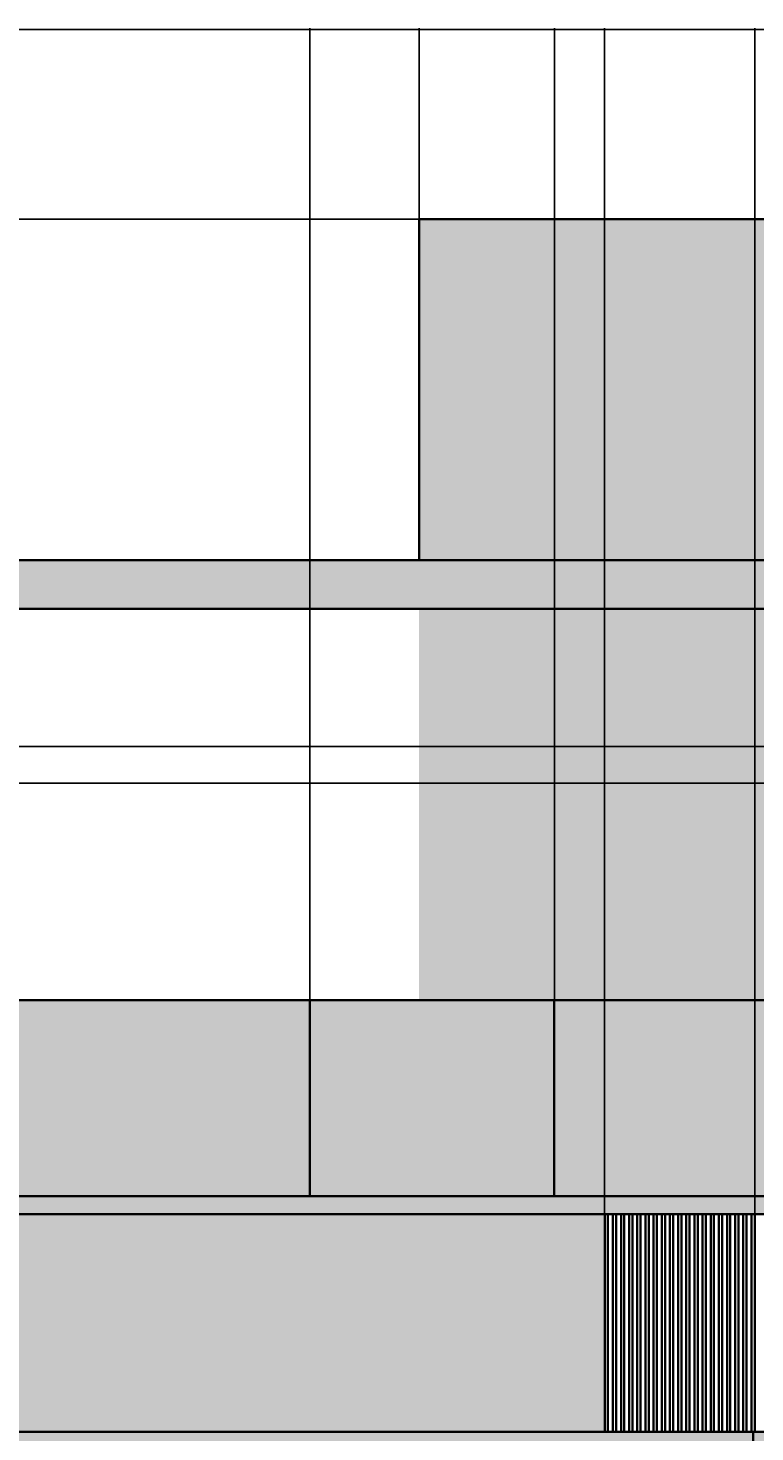
# Model space of a CAD drawing. Units: feet. Extents: x 2368 to 2738, y 1285 to 1782.
# Tile 4 of 6: x 2472 to 2561, y 1610 to 1782. Entities that reach past the tile are written whole.
import ezdxf

# ---------------------------------------------------------------- set-up
doc = ezdxf.new("R2010")
doc.units = ezdxf.units.FT
for name, color, linetype, lineweight in [('A-ANNO-DIMS', 2, 'Continuous', 18), ('A-ELEV', 7, 'Continuous', 35), ('A-ELEV-PATT', 252, 'Continuous', 13)]:
    doc.layers.add(name, color=color, linetype=linetype, lineweight=lineweight)
doc.styles.get("Standard").update_dxf_attribs({"font": 'arial.ttf'})
doc.dimstyles.get("Standard").update_dxf_attribs({"dimtxt": 0.18, "dimasz": 0.18, "dimexe": 0.18, "dimexo": 0.0625, "dimgap": 0.09, "dimtad": 0, "dimtih": 1, "dimtoh": 1, "dimdec": 1, "dimzin": 0, "dimdsep": 46, "dimlunit": 3, "dimtxsty": 'Standard', "dimcen": 0.09, "dimadec": 0, "dimazin": 0, "dimtfac": 1, "dimtdec": 1, "dimtofl": 0, "dimtmove": 0, "dimatfit": 3, "dimfxl": 1, "dimtolj": 1, "dimtzin": 0, "dimarcsym": 0})

# ---------------------------------------------------------------- blocks, each defined once
blk = doc.blocks.new('*D1')
at = {"layer": 'A-ANNO-DIMS', "color": 0, "lineweight": -2, "transparency": 16777216}
for p, q in [((2391.54, 1662.92), (2391.54, 1782.11)), ((2391.72, 1781.93), (2552.46, 1781.93)), ((2713.98, 1781.93), (2553.25, 1781.93)), ((2714.16, 1758.74), (2714.16, 1782.11))]:
    blk.add_line(p, q, dxfattribs=at)
at = {"layer": 'A-ANNO-DIMS', "color": 0, "transparency": 16777216}
for points in [[(2391.72, 1781.96), (2391.72, 1781.9), (2391.54, 1781.93)], [(2713.98, 1781.96), (2713.98, 1781.9), (2714.16, 1781.93)]]:
    blk.add_solid(points, dxfattribs=at)
at = {"layer": 'Defpoints', "color": 0, "transparency": 16777216}
for p in [(2714.16, 1781.93), (2714.16, 1758.68), (2391.54, 1662.86)]:
    blk.add_point(p, dxfattribs=at)
at = {"layer": 'A-ANNO-DIMS', "color": 0, "transparency": 16777216, "insert": (2552.85, 1781.93), "char_height": 0.18, "attachment_point": 5}
blk.add_mtext('\\A1;322.6', dxfattribs=at)
blk = doc.blocks.new('*D13')
at = {"layer": 'A-ANNO-DIMS', "color": 0, "lineweight": -2, "transparency": 16777216}
for p, q in [((2519.56, 1758.68), (2368.11, 1758.68)), ((2368.29, 1758.5), (2368.29, 1737.95)), ((2368.29, 1717.04), (2368.29, 1737.58)), ((2519.56, 1716.86), (2368.11, 1716.86))]:
    blk.add_line(p, q, dxfattribs=at)
at = {"layer": 'A-ANNO-DIMS', "color": 0, "transparency": 16777216}
for points in [[(2368.26, 1758.5), (2368.32, 1758.5), (2368.29, 1758.68)], [(2368.26, 1717.04), (2368.32, 1717.04), (2368.29, 1716.86)]]:
    blk.add_solid(points, dxfattribs=at)
at = {"layer": 'Defpoints', "color": 0, "transparency": 16777216}
for p in [(2368.29, 1758.68), (2519.62, 1758.68), (2519.62, 1716.86)]:
    blk.add_point(p, dxfattribs=at)
at = {"layer": 'A-ANNO-DIMS', "color": 0, "transparency": 16777216, "insert": (2368.29, 1737.77), "char_height": 0.18, "attachment_point": 5}
blk.add_mtext('\\A1;41.82', dxfattribs=at)
blk = doc.blocks.new('*D38')
at = {"layer": 'A-ANNO-DIMS', "color": 0, "lineweight": -2, "transparency": 16777216}
for p, q in [((2701.6, 1636.62), (2368.11, 1636.62)), ((2368.29, 1636.44), (2368.29, 1623.45)), ((2368.29, 1610.09), (2368.29, 1623.08)), ((2701.6, 1609.91), (2368.11, 1609.91))]:
    blk.add_line(p, q, dxfattribs=at)
at = {"layer": 'A-ANNO-DIMS', "color": 0, "transparency": 16777216}
for points in [[(2368.26, 1636.44), (2368.32, 1636.44), (2368.29, 1636.62)], [(2368.26, 1610.09), (2368.32, 1610.09), (2368.29, 1609.91)]]:
    blk.add_solid(points, dxfattribs=at)
at = {"layer": 'Defpoints', "color": 0, "transparency": 16777216}
for p in [(2368.29, 1636.62), (2701.66, 1636.62), (2701.66, 1609.91)]:
    blk.add_point(p, dxfattribs=at)
at = {"layer": 'A-ANNO-DIMS', "color": 0, "transparency": 16777216, "insert": (2368.29, 1623.26), "char_height": 0.18, "attachment_point": 5}
blk.add_mtext('\\A1;26.72', dxfattribs=at)
blk = doc.blocks.new('*D39')
at = {"layer": 'A-ANNO-DIMS', "color": 0, "lineweight": -2, "transparency": 16777216}
for p, q in [((2701.6, 1662.86), (2368.11, 1662.86)), ((2368.29, 1662.68), (2368.29, 1651.02)), ((2368.29, 1638.99), (2368.29, 1650.65)), ((2701.6, 1638.81), (2368.11, 1638.81))]:
    blk.add_line(p, q, dxfattribs=at)
at = {"layer": 'A-ANNO-DIMS', "color": 0, "transparency": 16777216}
for points in [[(2368.26, 1662.68), (2368.32, 1662.68), (2368.29, 1662.86)], [(2368.26, 1638.99), (2368.32, 1638.99), (2368.29, 1638.81)]]:
    blk.add_solid(points, dxfattribs=at)
at = {"layer": 'Defpoints', "color": 0, "transparency": 16777216}
for p in [(2368.29, 1662.86), (2701.66, 1662.86), (2701.66, 1638.81)]:
    blk.add_point(p, dxfattribs=at)
at = {"layer": 'A-ANNO-DIMS', "color": 0, "transparency": 16777216, "insert": (2368.29, 1650.83), "char_height": 0.18, "attachment_point": 5}
blk.add_mtext('\\A1;24.042', dxfattribs=at)
blk = doc.blocks.new('*D40')
at = {"layer": 'A-ANNO-DIMS', "color": 0, "lineweight": -2, "transparency": 16777216}
for p, q in [((2701.6, 1693.98), (2368.11, 1693.98)), ((2368.29, 1693.8), (2368.29, 1678.6)), ((2368.29, 1663.04), (2368.29, 1678.24)), ((2701.6, 1662.86), (2368.11, 1662.86))]:
    blk.add_line(p, q, dxfattribs=at)
at = {"layer": 'A-ANNO-DIMS', "color": 0, "transparency": 16777216}
for points in [[(2368.26, 1693.8), (2368.32, 1693.8), (2368.29, 1693.98)], [(2368.26, 1663.04), (2368.32, 1663.04), (2368.29, 1662.86)]]:
    blk.add_solid(points, dxfattribs=at)
at = {"layer": 'Defpoints', "color": 0, "transparency": 16777216}
for p in [(2368.29, 1693.98), (2701.66, 1693.98), (2701.66, 1662.86)]:
    blk.add_point(p, dxfattribs=at)
at = {"layer": 'A-ANNO-DIMS', "color": 0, "transparency": 16777216, "insert": (2368.29, 1678.42), "char_height": 0.18, "attachment_point": 5}
blk.add_mtext('\\A1;31.13', dxfattribs=at)
blk = doc.blocks.new('*D53')
at = {"layer": 'A-ANNO-DIMS', "color": 0, "lineweight": -2, "transparency": 16777216}
for p, q in [((2441.25, 1609.97), (2441.25, 1782.11)), ((2441.43, 1781.93), (2500.56, 1781.93)), ((2560.6, 1781.93), (2501.47, 1781.93)), ((2560.78, 1609.97), (2560.78, 1782.11))]:
    blk.add_line(p, q, dxfattribs=at)
at = {"layer": 'A-ANNO-DIMS', "color": 0, "transparency": 16777216}
for points in [[(2441.43, 1781.96), (2441.43, 1781.9), (2441.25, 1781.93)], [(2560.6, 1781.96), (2560.6, 1781.9), (2560.78, 1781.93)]]:
    blk.add_solid(points, dxfattribs=at)
at = {"layer": 'Defpoints', "color": 0, "transparency": 16777216}
for p in [(2560.78, 1781.93), (2441.25, 1609.91), (2560.78, 1609.91)]:
    blk.add_point(p, dxfattribs=at)
at = {"layer": 'A-ANNO-DIMS', "color": 0, "transparency": 16777216, "insert": (2501.01, 1781.93), "char_height": 0.18, "attachment_point": 5}
blk.add_mtext('\\A1;119.53', dxfattribs=at)
blk = doc.blocks.new('*D54')
at = {"layer": 'A-ANNO-DIMS', "color": 0, "lineweight": -2, "transparency": 16777216}
for p, q in [((2560.78, 1609.97), (2560.78, 1782.11)), ((2560.96, 1781.93), (2564.98, 1781.93)), ((2569.66, 1781.93), (2565.63, 1781.93)), ((2569.84, 1609.97), (2569.84, 1782.11))]:
    blk.add_line(p, q, dxfattribs=at)
at = {"layer": 'A-ANNO-DIMS', "color": 0, "transparency": 16777216}
for points in [[(2560.96, 1781.96), (2560.96, 1781.9), (2560.78, 1781.93)], [(2569.66, 1781.96), (2569.66, 1781.9), (2569.84, 1781.93)]]:
    blk.add_solid(points, dxfattribs=at)
at = {"layer": 'Defpoints', "color": 0, "transparency": 16777216}
for p in [(2569.84, 1781.93), (2560.78, 1609.91), (2569.84, 1609.91)]:
    blk.add_point(p, dxfattribs=at)
at = {"layer": 'A-ANNO-DIMS', "color": 0, "transparency": 16777216, "insert": (2565.31, 1781.93), "char_height": 0.18, "attachment_point": 5}
blk.add_mtext('\\A1;9.06', dxfattribs=at)
blk = doc.blocks.new('*D62')
at = {"layer": 'A-ANNO-DIMS', "color": 0, "lineweight": -2, "transparency": 16777216}
for p, q in [((2441.25, 1636.69), (2441.25, 1782.11)), ((2441.43, 1781.93), (2491.36, 1781.93)), ((2542.19, 1781.93), (2492.27, 1781.93)), ((2542.37, 1636.69), (2542.37, 1782.11))]:
    blk.add_line(p, q, dxfattribs=at)
at = {"layer": 'A-ANNO-DIMS', "color": 0, "transparency": 16777216}
for points in [[(2441.43, 1781.96), (2441.43, 1781.9), (2441.25, 1781.93)], [(2542.19, 1781.96), (2542.19, 1781.9), (2542.37, 1781.93)]]:
    blk.add_solid(points, dxfattribs=at)
at = {"layer": 'Defpoints', "color": 0, "transparency": 16777216}
for p in [(2542.37, 1781.93), (2441.25, 1636.62), (2542.37, 1636.62)]:
    blk.add_point(p, dxfattribs=at)
at = {"layer": 'A-ANNO-DIMS', "color": 0, "transparency": 16777216, "insert": (2491.81, 1781.93), "char_height": 0.18, "attachment_point": 5}
blk.add_mtext('\\A1;101.13', dxfattribs=at)
blk = doc.blocks.new('*D63')
at = {"layer": 'A-ANNO-DIMS', "color": 0, "lineweight": -2, "transparency": 16777216}
for p, q in [((2415.54, 1662.92), (2415.54, 1782.11)), ((2415.72, 1781.93), (2460.47, 1781.93)), ((2506.02, 1781.93), (2461.26, 1781.93)), ((2506.2, 1662.92), (2506.2, 1782.11))]:
    blk.add_line(p, q, dxfattribs=at)
at = {"layer": 'A-ANNO-DIMS', "color": 0, "transparency": 16777216}
for points in [[(2415.72, 1781.96), (2415.72, 1781.9), (2415.54, 1781.93)], [(2506.02, 1781.96), (2506.02, 1781.9), (2506.2, 1781.93)]]:
    blk.add_solid(points, dxfattribs=at)
at = {"layer": 'Defpoints', "color": 0, "transparency": 16777216}
for p in [(2506.2, 1781.93), (2415.54, 1662.86), (2506.2, 1662.86)]:
    blk.add_point(p, dxfattribs=at)
at = {"layer": 'A-ANNO-DIMS', "color": 0, "transparency": 16777216, "insert": (2460.87, 1781.93), "char_height": 0.18, "attachment_point": 5}
blk.add_mtext('\\A1;90.65', dxfattribs=at)
blk = doc.blocks.new('*D64')
at = {"layer": 'A-ANNO-DIMS', "color": 0, "lineweight": -2, "transparency": 16777216}
for p, q in [((2506.2, 1662.92), (2506.2, 1782.11)), ((2506.38, 1781.93), (2520.98, 1781.93)), ((2536.02, 1781.93), (2521.41, 1781.93)), ((2536.2, 1662.92), (2536.2, 1782.11))]:
    blk.add_line(p, q, dxfattribs=at)
at = {"layer": 'A-ANNO-DIMS', "color": 0, "transparency": 16777216}
for points in [[(2506.38, 1781.96), (2506.38, 1781.9), (2506.2, 1781.93)], [(2536.02, 1781.96), (2536.02, 1781.9), (2536.2, 1781.93)]]:
    blk.add_solid(points, dxfattribs=at)
at = {"layer": 'Defpoints', "color": 0, "transparency": 16777216}
for p in [(2536.2, 1781.93), (2506.2, 1662.86), (2536.2, 1662.86)]:
    blk.add_point(p, dxfattribs=at)
at = {"layer": 'A-ANNO-DIMS', "color": 0, "transparency": 16777216, "insert": (2521.2, 1781.93), "char_height": 0.18, "attachment_point": 5}
blk.add_mtext('\\A1;30', dxfattribs=at)
blk = doc.blocks.new('*D68')
at = {"layer": 'A-ANNO-DIMS', "color": 0, "lineweight": -2, "transparency": 16777216}
for p, q in [((2409.54, 1716.92), (2409.54, 1782.11)), ((2409.72, 1781.93), (2464.13, 1781.93)), ((2519.44, 1781.93), (2465.04, 1781.93)), ((2519.62, 1716.92), (2519.62, 1782.11))]:
    blk.add_line(p, q, dxfattribs=at)
at = {"layer": 'A-ANNO-DIMS', "color": 0, "transparency": 16777216}
for points in [[(2409.72, 1781.96), (2409.72, 1781.9), (2409.54, 1781.93)], [(2519.44, 1781.96), (2519.44, 1781.9), (2519.62, 1781.93)]]:
    blk.add_solid(points, dxfattribs=at)
at = {"layer": 'Defpoints', "color": 0, "transparency": 16777216}
for p in [(2519.62, 1781.93), (2409.54, 1716.86), (2519.62, 1716.86)]:
    blk.add_point(p, dxfattribs=at)
at = {"layer": 'A-ANNO-DIMS', "color": 0, "transparency": 16777216, "insert": (2464.58, 1781.93), "char_height": 0.18, "attachment_point": 5}
blk.add_mtext('\\A1;110.08', dxfattribs=at)
blk = doc.blocks.new('*D69')
at = {"layer": 'A-ANNO-DIMS', "color": 0, "lineweight": -2, "transparency": 16777216}
for p, q in [((2519.62, 1716.92), (2519.62, 1782.11)), ((2519.8, 1781.93), (2555.62, 1781.93)), ((2592.23, 1781.93), (2556.41, 1781.93)), ((2592.41, 1689.56), (2592.41, 1782.11))]:
    blk.add_line(p, q, dxfattribs=at)
at = {"layer": 'A-ANNO-DIMS', "color": 0, "transparency": 16777216}
for points in [[(2519.8, 1781.96), (2519.8, 1781.9), (2519.62, 1781.93)], [(2592.23, 1781.96), (2592.23, 1781.9), (2592.41, 1781.93)]]:
    blk.add_solid(points, dxfattribs=at)
at = {"layer": 'Defpoints', "color": 0, "transparency": 16777216}
for p in [(2592.41, 1781.93), (2519.62, 1716.86), (2592.41, 1689.49)]:
    blk.add_point(p, dxfattribs=at)
at = {"layer": 'A-ANNO-DIMS', "color": 0, "transparency": 16777216, "insert": (2556.02, 1781.93), "char_height": 0.18, "attachment_point": 5}
blk.add_mtext('\\A1;72.79', dxfattribs=at)
blk = doc.blocks.new('*D71')
at = {"layer": 'A-ANNO-DIMS', "color": 0, "lineweight": -2, "transparency": 16777216}
for p, q in [((2592.35, 1689.49), (2368.11, 1689.49)), ((2368.29, 1689.31), (2368.29, 1676.36)), ((2368.29, 1663.04), (2368.29, 1675.99)), ((2592.35, 1662.86), (2368.11, 1662.86))]:
    blk.add_line(p, q, dxfattribs=at)
at = {"layer": 'A-ANNO-DIMS', "color": 0, "transparency": 16777216}
for points in [[(2368.26, 1689.31), (2368.32, 1689.31), (2368.29, 1689.49)], [(2368.26, 1663.04), (2368.32, 1663.04), (2368.29, 1662.86)]]:
    blk.add_solid(points, dxfattribs=at)
at = {"layer": 'Defpoints', "color": 0, "transparency": 16777216}
for p in [(2368.29, 1689.49), (2592.41, 1689.49), (2592.41, 1662.86)]:
    blk.add_point(p, dxfattribs=at)
at = {"layer": 'A-ANNO-DIMS', "color": 0, "transparency": 16777216, "insert": (2368.29, 1676.17), "char_height": 0.18, "attachment_point": 5}
blk.add_mtext('\\A1;26.64', dxfattribs=at)

msp = doc.modelspace()

# ---------------------------------------------------------------- hatches: boundary and pattern name
at = {"layer": 'A-ELEV-PATT'}
h = msp.add_hatch(color=256, dxfattribs=at)
h.set_gradient(color1=(192, 192, 192), color2=(192, 192, 192), tint=1)
h.paths.add_polyline_path([(2714.1625, 1758.6751), (2519.621, 1758.6751), (2519.621, 1716.8552), (2714.1625, 1716.8552)])
h.paths.add_polyline_path([(2701.6591, 1693.9847), (2714.1625, 1693.9847), (2714.1625, 1710.8552), (2519.621, 1710.8552), (2519.621, 1662.8552), (2592.4132, 1662.8552), (2592.4132, 1689.493), (2665.1962, 1689.493), (2665.1962, 1662.8552), (2701.6591, 1662.8552)])
h.paths.add_polyline_path([(2701.6591, 1609.9058), (2597.776, 1609.9058), (2597.776, 1600.4784), (2665.1962, 1600.4784), (2665.1962, 1596.3371), (2665.1962, 1522.6314), (2701.6591, 1522.6314)])
h.paths.add_polyline_path([(2463.0324, 1598.097), (2536.677, 1598.097), (2536.677, 1519.7115), (2560.74, 1519.7115), (2560.5754, 1609.9058), (2542.3749, 1609.9058), (2441.2488, 1609.9058), (2441.2488, 1519.7115), (2463.0324, 1519.7115)])
h.paths.add_polyline_path([(2506.1956, 1662.8552), (2391.5414, 1662.8552), (2391.5414, 1644.4206), (2438.815, 1644.4206, -0.34592239), (2445.9507, 1638.8128), (2506.1956, 1638.8128)])
h.paths.add_polyline_path([(2410.9473, 1609.9058, -0.04175491), (2411.9608, 1614.8552), (2391.5414, 1614.8552), (2391.5414, 1488.8552), (2410.9473, 1488.8552)])
h.paths.add_polyline_path([(2426.5897, 1605.0962, 1), (2422.7862, 1605.0962), (2422.7862, 1509.5049, 1), (2426.5897, 1509.5049)])
h.paths.add_polyline_path([(2463.0324, 1460.097), (2536.677, 1460.097), (2536.677, 1350.8552), (2543.4468, 1350.8552), (2543.4468, 1482.8552), (2391.5414, 1482.8552), (2391.5414, 1350.8552), (2463.0324, 1350.8552)])
h.paths.add_polyline_path([(2436.8485, 1456.084), (2436.8485, 1379.669), (2399.9065, 1379.669), (2399.9065, 1456.084)], flags=16)
h.paths.add_polyline_path([(2434.8485, 1454.084), (2434.8485, 1381.669), (2401.9065, 1381.669), (2401.9065, 1454.084)], flags=0)
h.paths.add_polyline_path([(2714.1625, 1350.8552), (2391.5414, 1350.8552), (2391.5414, 1320.8552), (2714.1625, 1320.8552)])
h.paths.add_polyline_path([(2714.1625, 1320.8552), (2391.5414, 1320.8552), (2391.5414, 1308.8552), (2714.1625, 1308.8552)])
h = msp.add_hatch(color=256, dxfattribs=at)
h.set_gradient(color1=(128, 128, 128), color2=(128, 128, 128), tint=1)
h.paths.add_polyline_path([(2519.621, 1716.8552), (2409.5414, 1716.8552), (2409.5414, 1662.8552), (2415.5414, 1662.8552), (2415.5414, 1710.8552), (2519.621, 1710.8552)])
h.paths.add_polyline_path([(2714.1625, 1716.8552), (2519.621, 1716.8552), (2519.621, 1710.8552), (2714.1625, 1710.8552)])
h.paths.add_polyline_path([(2701.6591, 1638.8128), (2445.9507, 1638.8128, -0.0752442), (2446.1448, 1636.6235), (2542.3749, 1636.6235), (2542.776, 1636.6235), (2701.6591, 1636.6235)])
h = msp.add_hatch(color=256, dxfattribs=at)
h.set_gradient(color1=(255, 255, 255), tint=1)
h.paths.add_polyline_path([(2595.4132, 1686.493), (2662.1962, 1686.493), (2662.1962, 1662.8552), (2665.1962, 1662.8552), (2665.1962, 1689.493), (2592.4132, 1689.493), (2592.4132, 1662.8552), (2595.4132, 1662.8552)])
h.paths.add_polyline_path([(2665.1962, 1600.4784), (2597.776, 1600.4784), (2597.776, 1597.4784), (2662.1962, 1597.4784), (2662.1962, 1510.3225), (2597.776, 1510.3225), (2597.776, 1507.3225), (2665.1962, 1507.3225)])
h.paths.add_polyline_path([(2665.1962, 1461.1396), (2592.4132, 1461.1396), (2592.4132, 1367.9838), (2665.1962, 1367.9838)])
h.paths.add_polyline_path([(2662.1962, 1458.1396), (2662.1962, 1370.9838), (2595.4132, 1370.9838), (2595.4132, 1458.1396)], flags=16)
h.paths.add_polyline_path([(2593.776, 1609.9058), (2584.2358, 1609.9058), (2584.2358, 1488.8552), (2593.776, 1488.8552)])
h.paths.add_polyline_path([(2597.776, 1609.9058), (2595.4517, 1609.9058), (2595.4517, 1488.8552), (2597.776, 1488.8552)])
h.paths.add_polyline_path([(2569.8357, 1609.9058), (2560.5754, 1609.9058), (2560.74, 1519.7115), (2560.7407, 1519.7115), (2560.7407, 1519.3328), (2560.7963, 1488.8552), (2569.8357, 1488.8552)])
h.paths.add_polyline_path([(2572.6807, 1609.9058), (2571.6967, 1609.9058), (2571.6967, 1488.8552), (2572.6807, 1488.8552)])
h.paths.add_polyline_path([(2575.8428, 1609.9058), (2574.5416, 1609.9058), (2574.5416, 1488.8552), (2575.8428, 1488.8552)])
h.paths.add_polyline_path([(2579.0308, 1609.9058), (2577.7037, 1609.9058), (2577.7037, 1488.8552), (2579.0308, 1488.8552)])
h.paths.add_polyline_path([(2582.3749, 1609.9058), (2580.8918, 1609.9058), (2580.8918, 1488.8552), (2582.3749, 1488.8552)])
h = msp.add_hatch(color=256, dxfattribs=at)
h.set_gradient(color1=(153, 185, 219), color2=(153, 185, 219), tint=1)
h.paths.add_polyline_path([(2536.1956, 1662.8552), (2506.1956, 1662.8552), (2506.1956, 1638.8128), (2536.1956, 1638.8128)])
h.paths.add_polyline_path([(2566.1956, 1662.8552), (2536.1956, 1662.8552), (2536.1956, 1638.8128), (2566.1956, 1638.8128)])
h.paths.add_polyline_path([(2596.1956, 1662.8552), (2566.1956, 1662.8552), (2566.1956, 1638.8128), (2596.1956, 1638.8128)])
h.paths.add_polyline_path([(2626.1956, 1662.8552), (2596.1956, 1662.8552), (2596.1956, 1638.8128), (2626.1956, 1638.8128)])
h.paths.add_polyline_path([(2656.1956, 1662.8552), (2626.1956, 1662.8552), (2626.1956, 1638.8128), (2656.1956, 1638.8128)])
h.paths.add_polyline_path([(2686.1956, 1662.8552), (2656.1956, 1662.8552), (2656.1956, 1638.8128), (2686.1956, 1638.8128)])
h.paths.add_polyline_path([(2701.6591, 1662.8552), (2686.1956, 1662.8552), (2686.1956, 1638.8128), (2701.6591, 1638.8128)])
h = msp.add_hatch(color=256, dxfattribs=at)
h.set_gradient(color1=(242, 242, 242), color2=(242, 242, 242), tint=1)
h.paths.add_polyline_path([(2542.3749, 1636.6235), (2440.8236, 1636.6235, 0.37790365), (2410.9473, 1609.9058), (2410.9473, 1488.8552), (2441.2488, 1488.8552), (2441.2488, 1609.9058), (2542.3749, 1609.9058)])
h.paths.add_polyline_path([(2426.5897, 1605.0962), (2426.5897, 1509.5049, -1), (2422.7862, 1509.5049), (2422.7862, 1605.0962, -1)], flags=16)
h.paths.add_polyline_path([(2441.2488, 1636.6235), (2446.1448, 1636.6235, 0.43242195), (2438.815, 1644.4206), (2391.5414, 1644.4206), (2391.5414, 1620.8552), (2391.5414, 1614.8552), (2411.9608, 1614.8552, -0.33482359)])
h.paths.add_polyline_path([(2592.4132, 1461.1396), (2635.4878, 1461.1396), (2635.4878, 1466.101), (2560.7963, 1466.101), (2560.7963, 1482.8552), (2543.4468, 1482.8552), (2543.4468, 1350.8552), (2635.4878, 1350.8552), (2635.4878, 1367.9838), (2592.4132, 1367.9838)])

# ---------------------------------------------------------------- linework, layer by layer
at = {"layer": 'A-ELEV'}
for p, q in [((2519.621, 1758.6751), (2714.1625, 1758.6751)), ((2714.1625, 1758.6751), (2519.621, 1758.6751)), ((2519.621, 1758.6751), (2519.621, 1716.8552)), ((2409.5414, 1716.8552), (2714.1625, 1716.8552)), ((2519.621, 1716.8552), (2714.1625, 1716.8552)), ((2415.5414, 1710.8552), (2714.1625, 1710.8552)), ((2519.662, 1710.8552), (2714.1625, 1710.8552)), ((2391.5414, 1662.8552), (2701.6591, 1662.8552)), ((2701.6591, 1662.8552), (2391.5414, 1662.8552)), ((2506.1956, 1662.8552), (2506.1956, 1638.8128)), ((2506.1956, 1638.8128), (2506.1956, 1662.8552)), ((2506.1956, 1662.8552), (2519.326, 1662.8552)), ((2536.1956, 1662.8552), (2536.1956, 1638.8128)), ((2536.1956, 1638.8128), (2536.1956, 1662.8552)), ((2445.9507, 1638.8128), (2701.6591, 1638.8128)), ((2445.9507, 1638.8128), (2701.6591, 1638.8128)), ((2446.1448, 1636.6235), (2701.6591, 1636.6235)), ((2542.3749, 1636.6235), (2701.6591, 1636.6235)), ((2441.2488, 1609.9058), (2701.6591, 1609.9058)), ((2542.3749, 1609.9058), (2701.6591, 1609.9058)), ((2560.7963, 1488.8552), (2560.5754, 1609.9058))]:
    msp.add_line(p, q, dxfattribs=at)
msp.add_lwpolyline([(2441.2488, 1609.9058), (2542.3749, 1609.9058), (2542.3749, 1636.6235), (2441.2488, 1636.6235)], dxfattribs=at)
for points in [[(2542.3749, 1636.6235), (2542.776, 1636.6235), (2542.776, 1609.9058), (2542.3749, 1609.9058)], [(2543.3749, 1636.6235), (2543.776, 1636.6235), (2543.776, 1609.9058), (2543.3749, 1609.9058)], [(2544.3749, 1636.6235), (2544.776, 1636.6235), (2544.776, 1609.9058), (2544.3749, 1609.9058)], [(2545.3749, 1636.6235), (2545.776, 1636.6235), (2545.776, 1609.9058), (2545.3749, 1609.9058)], [(2546.3749, 1636.6235), (2546.776, 1636.6235), (2546.776, 1609.9058), (2546.3749, 1609.9058)], [(2547.3749, 1636.6235), (2547.776, 1636.6235), (2547.776, 1609.9058), (2547.3749, 1609.9058)], [(2548.3749, 1636.6235), (2548.776, 1636.6235), (2548.776, 1609.9058), (2548.3749, 1609.9058)], [(2549.3749, 1636.6235), (2549.776, 1636.6235), (2549.776, 1609.9058), (2549.3749, 1609.9058)], [(2550.3749, 1636.6235), (2550.776, 1636.6235), (2550.776, 1609.9058), (2550.3749, 1609.9058)], [(2551.3749, 1636.6235), (2551.776, 1636.6235), (2551.776, 1609.9058), (2551.3749, 1609.9058)], [(2552.3749, 1636.6235), (2552.776, 1636.6235), (2552.776, 1609.9058), (2552.3749, 1609.9058)], [(2553.3749, 1636.6235), (2553.776, 1636.6235), (2553.776, 1609.9058), (2553.3749, 1609.9058)], [(2554.3749, 1636.6235), (2554.776, 1636.6235), (2554.776, 1609.9058), (2554.3749, 1609.9058)], [(2555.3749, 1636.6235), (2555.776, 1636.6235), (2555.776, 1609.9058), (2555.3749, 1609.9058)], [(2556.3749, 1636.6235), (2556.776, 1636.6235), (2556.776, 1609.9058), (2556.3749, 1609.9058)], [(2557.3749, 1636.6235), (2557.776, 1636.6235), (2557.776, 1609.9058), (2557.3749, 1609.9058)], [(2558.3749, 1636.6235), (2558.776, 1636.6235), (2558.776, 1609.9058), (2558.3749, 1609.9058)], [(2559.3749, 1636.6235), (2559.776, 1636.6235), (2559.776, 1609.9058), (2559.3749, 1609.9058)], [(2560.3749, 1636.6235), (2560.776, 1636.6235), (2560.776, 1609.9058), (2560.3749, 1609.9058)]]:
    msp.add_lwpolyline(points, close=True, dxfattribs=at)

# ---------------------------------------------------------------- dimensions: what is measured, and where the dimension line sits
at = {"layer": 'A-ANNO-DIMS'}
for base, p1, p2, override, picture, middle in [((2714.1625, 1781.9251), (2391.5414, 1662.8552), (2714.1625, 1758.6751), {"dimdec": 1, "dimlfac": 1, "dimrnd": 0, "dimzin": 0, "dimdsep": 46, "dimlunit": 2}, '*D1', (2552.8519, 1781.9251)), ((2519.621, 1781.9251), (2409.5414, 1716.8552), (2519.621, 1716.8552), {"dimdec": 2, "dimlfac": 1, "dimrnd": 0, "dimzin": 0, "dimdsep": 46, "dimlunit": 2}, '*D68', (2464.5812, 1781.9251)), ((2506.1956, 1781.9251), (2415.5414, 1662.8552), (2506.1956, 1662.8552), {"dimdec": 2, "dimlfac": 1, "dimrnd": 0, "dimzin": 0, "dimdsep": 46, "dimlunit": 2}, '*D63', (2460.8685, 1781.9251)), ((2560.776, 1781.9251), (2441.2488, 1609.9058), (2560.776, 1609.9058), {"dimdec": 2, "dimlfac": 1, "dimrnd": 0, "dimzin": 0, "dimdsep": 46, "dimlunit": 2}, '*D53', (2501.0124, 1781.9251)), ((2542.3749, 1781.9251), (2441.2488, 1636.6235), (2542.3749, 1636.6235), {"dimdec": 2, "dimlfac": 1, "dimrnd": 0, "dimzin": 0, "dimdsep": 46, "dimlunit": 2}, '*D62', (2491.8118, 1781.9251)), ((2536.1956, 1781.9251), (2506.1956, 1662.8552), (2536.1956, 1662.8552), {"dimdec": 0, "dimlfac": 1, "dimrnd": 0, "dimzin": 0, "dimdsep": 46, "dimlunit": 2}, '*D64', (2521.1956, 1781.9251)), ((2592.4132, 1781.9251), (2519.621, 1716.8552), (2592.4132, 1689.493), {"dimdec": 2, "dimlfac": 1, "dimrnd": 0, "dimzin": 0, "dimdsep": 46, "dimlunit": 2}, '*D69', (2556.0171, 1781.9251)), ((2569.8357, 1781.9251), (2560.776, 1609.9058), (2569.8357, 1609.9058), {"dimdec": 2, "dimlfac": 1, "dimrnd": 0, "dimzin": 0, "dimdsep": 46, "dimlunit": 2}, '*D54', (2565.3059, 1781.9251))]:
    dim = msp.add_linear_dim(base=base, p1=p1, p2=p2, dimstyle='Standard', override=override, dxfattribs=at)
    dim.commit()
    dim.dimension.update_dxf_attribs({"geometry": picture, "text_midpoint": middle})
for base, p1, p2, override, picture, middle in [((2368.2914, 1758.6751), (2519.621, 1716.8552), (2519.621, 1758.6751), {"dimdec": 2, "dimlfac": 1, "dimrnd": 0, "dimzin": 0, "dimdsep": 46, "dimlunit": 2}, '*D13', (2368.2914, 1737.7652)), ((2368.2914, 1693.9847), (2701.6591, 1662.8552), (2701.6591, 1693.9847), {"dimdec": 2, "dimlfac": 1, "dimrnd": 0, "dimzin": 0, "dimdsep": 46, "dimlunit": 2}, '*D40', (2368.2914, 1678.42)), ((2368.2914, 1689.493), (2592.4132, 1662.8552), (2592.4132, 1689.493), {"dimdec": 2, "dimlfac": 1, "dimrnd": 0, "dimzin": 0, "dimdsep": 46, "dimlunit": 2}, '*D71', (2368.2914, 1676.1741)), ((2368.2914, 1662.8552), (2701.6591, 1638.8128), (2701.6591, 1662.8552), {"dimdec": 3, "dimlfac": 1, "dimrnd": 0, "dimzin": 0, "dimdsep": 46, "dimlunit": 2}, '*D39', (2368.2914, 1650.834)), ((2368.2914, 1636.6235), (2701.6591, 1609.9058), (2701.6591, 1636.6235), {"dimdec": 2, "dimlfac": 1, "dimrnd": 0, "dimzin": 0, "dimdsep": 46, "dimlunit": 2}, '*D38', (2368.2914, 1623.2646))]:
    dim = msp.add_linear_dim(base=base, p1=p1, p2=p2, angle=90, dimstyle='Standard', override=override, dxfattribs=at)
    dim.commit()
    dim.dimension.update_dxf_attribs({"geometry": picture, "text_midpoint": middle})

doc.saveas('drawing.dxf')
